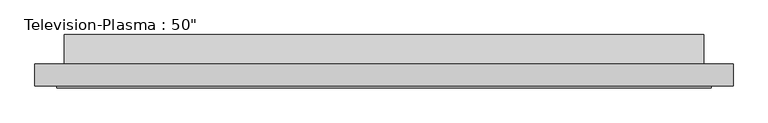
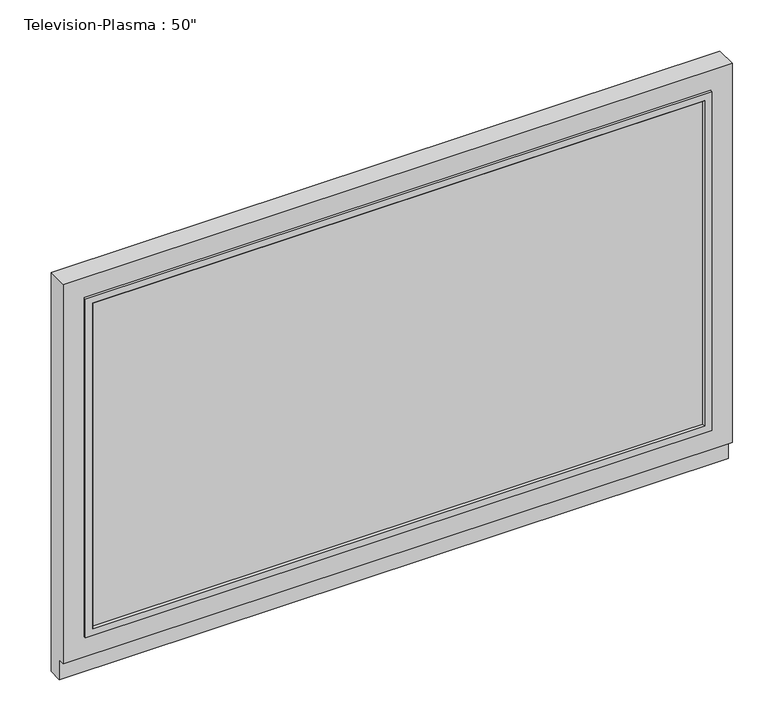
"""IFC4 building model written with IfcOpenShell, lengths in millimetres: furniture geometry."""

from ifc_helpers import new_model, si_unit, frame, origin, place, context, project, spatial, polyline, outline, extrude, faceted_brep, source, transform, mapped, element, save


def furniture_5e39d705(model_context):
    return source(origin(), model_context, "Body", "SolidModel", [
        extrude(outline(polyline([(609.6, -88.9), (-495.3, -88.9), (-495.3, -74.1720413), (609.6, -74.1720413), (609.6, -88.9)])), frame((0.0, 0.0, 88.9), z_axis=(0.0, 0.0, 1.0), x_axis=(1.0, 0.0, 0.0)), (0.0, 0.0, 1.0), 622.3),
        faceted_brep([(660.4, -50.8, 762.0), (-546.1, -50.8, 762.0), (-546.1, -88.9, 762.0), (660.4, -88.9, 762.0), (-546.1, -50.8, 0.0), (660.4, -50.8, 0.0), (660.4, -76.2, 0.0), (-546.1, -76.2, 0.0), (-495.3, -50.8, 711.2), (-495.3, -50.8, 38.1), (609.6, -50.8, 38.1), (609.6, -50.8, 711.2), (-546.1, -76.2, 38.1), (-546.1, -88.9, 38.1), (660.4, -88.9, 38.1), (-508.0, -88.9, 723.9), (622.3, -88.9, 723.9), (622.3, -88.9, 723.10625), (622.3, -88.9, 76.2), (-508.0, -88.9, 76.2), (-508.0, -88.9, 723.10625), (660.4, -76.2, 38.1), (622.3, -74.1720413, 723.9), (-508.0, -74.1720413, 723.9), (-508.0, -74.1720413, 723.10625), (622.3, -74.1720413, 723.10625), (609.6, -74.1720413, 88.9), (609.6, -74.1720413, 710.40625), (-495.3, -74.1720413, 710.40625), (-495.3, -74.1720413, 88.9), (-495.3, 0.0, 676.4688953), (-495.3, 0.0, 38.1), (609.6, 0.0, 676.4688953), (609.6, 0.0, 38.1), (606.425, -88.9, 92.075), (609.6, -92.075, 88.9), (609.6, -92.075, 710.40625), (606.425, -88.9, 707.23125), (609.6, -88.9, 88.9), (609.6, -88.9, 710.40625), (622.3, -92.075, 723.10625), (622.3, -92.075, 76.2), (-495.3, -92.075, 710.40625), (-492.125, -88.9, 707.23125), (-495.3, -88.9, 710.40625), (-508.0, -92.075, 723.10625), (-495.3, -92.075, 88.9), (-492.125, -88.9, 92.075), (-495.3, -88.9, 88.9), (-508.0, -92.075, 76.2)], [[[0, 1, 2, 3]], [[4, 5, 6, 7]], [[1, 0, 5, 4], [8, 9, 10, 11]], [[2, 1, 4, 7, 12, 13]], [[3, 2, 13, 14], [15, 16, 17, 18, 19, 20]], [[0, 3, 14, 21, 6, 5]], [[22, 23, 24, 25]], [[26, 27, 28, 29]], [[16, 22, 25, 17]], [[23, 15, 20, 24]], [[23, 22, 16, 15]], [[21, 12, 7, 6]], [[12, 21, 14, 13]], [[30, 31, 9, 8]], [[32, 11, 10, 33]], [[31, 30, 32, 33]], [[9, 31, 33, 10]], [[30, 8, 11, 32]], [[34, 35, 36, 37]], [[26, 38, 39, 27]], [[40, 41, 18, 17]], [[37, 36, 42, 43]], [[27, 39, 44, 28]], [[45, 40, 17, 25, 24, 20]], [[43, 42, 46, 47]], [[28, 44, 48, 29]], [[49, 45, 20, 19]], [[41, 40, 45, 49], [36, 35, 46, 42]], [[35, 34, 47, 46]], [[39, 38, 48, 44], [34, 37, 43, 47]], [[38, 26, 29, 48]], [[41, 49, 19, 18]]]),
    ])


if __name__ == "__main__":
    model = new_model("IFC4")
    model_context = context("Model", 3, world=origin())
    ifc_project = project(units=[si_unit("LENGTHUNIT", "METRE", prefix="MILLI")], contexts=[model_context])
    site = spatial("IfcSite", under=ifc_project)
    building = spatial("IfcBuilding", under=site)
    placement = place(None, origin())
    furniture_shape = furniture_5e39d705(model_context)
    element("IfcFurniture", 1, ObjectType="Television-Plasma : 50\"", at=placement, inside=building, context=model_context, shape_type="MappedRepresentation", body=[
        mapped(furniture_shape, transform((0.0, 0.0, 0.0), x_axis=(1.0, 0.0, 0.0), y_axis=(0.0, 1.0, 0.0), z_axis=(0.0, 0.0, 1.0))),
    ])
    save(model, "model.ifc")

# Revit data of these elements
# Type "Television-Plasma : 50\""
#   Assembly Code = "E2020200"
#   Depth = 0' - 3 1/2"
#   Height = 2' - 6"
#   Width = 3' - 11 1/2"
#   Cabinet Material = Plastic - Gray
#   Default Elevation = 0
# Element 1 (IfcFurniture, "Television-Plasma : 50\"")
#   Materials on its faces: "Plastic - Gray", "Glass"
# Materials
#   "Plastic - Gray": colour RGB 134 134 134, transparency 0
#   "Glass": class "Glass", colour RGB 0 128 192, transparency 0.75, Description = "Soda Lime Glass", Cost = 0
